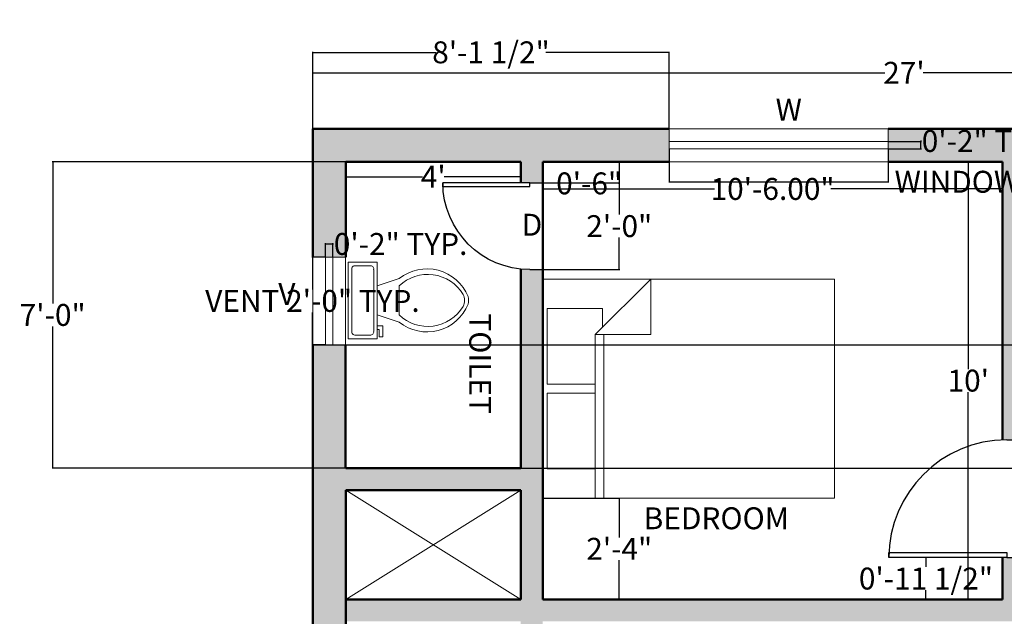
# Model space of a CAD drawing. Units: inches. Extents: x -53 to 395, y -10 to 410.
# Tile 2 of 3: x -53 to 217, y 247 to 410. Entities that reach past the tile are written whole.
import ezdxf

# ---------------------------------------------------------------- set-up
doc = ezdxf.new("R2010")
doc.units = ezdxf.units.IN
doc.header["$MEASUREMENT"] = 0
for name, color, linetype, lineweight in [('A-ANNO-DIMS', 2, 'Continuous', 18), ('A-ANNO-TEXT', 7, 'Continuous', 18), ('A-AREA-IDEN', 7, 'Continuous', 25), ('A-DOOR', 4, 'Continuous', 25), ('A-FLOR-FIXT', 9, 'Continuous', 20), ('A-FLOR-OPEN', 7, 'Continuous', 18), ('A-FURN', 8, 'Continuous', 18), ('A-GLAZ', 5, 'Continuous', 18), ('A-WALL', 7, 'Continuous', 50)]:
    doc.layers.add(name, color=color, linetype=linetype, lineweight=lineweight)
doc.layers.add('A-WALL-PATT', color=219, linetype='Continuous', lineweight=13, true_color=0x642165)
doc.styles.get("Standard").update_dxf_attribs({"font": 'arial.ttf'})
doc.dimstyles.get("Standard").update_dxf_attribs({"dimtxt": 6, "dimasz": 0.18, "dimexe": 0.18, "dimexo": 0.0625, "dimgap": 0.09, "dimtad": 0, "dimtih": 1, "dimtoh": 1, "dimzin": 0, "dimdsep": 46, "dimlunit": 3, "dimtxsty": 'Standard', "dimcen": 0.09, "dimadec": 0, "dimazin": 0, "dimtfac": 1, "dimtofl": 0, "dimtmove": 0, "dimatfit": 3, "dimfxl": 1, "dimtolj": 1, "dimtzin": 0, "dimarcsym": 0})

# ---------------------------------------------------------------- blocks, each defined once
blk = doc.blocks.new('*U2')
for p, q in [((0, 0), (0, -6)), ((40, 0), (40, -6))]:
    blk.add_line(p, q)
blk.add_lwpolyline([(0, 0), (0, 40), (1.75, 40), (1.75, 0)], close=True)
blk.add_arc((0, 0), 40, 0, 90)
blk = doc.blocks.new('Bed - Queen')
for p, q in [((0, -80.00003), (0, 0)), ((0, 0), (59.99999, 0)), ((59.99999, 0), (59.99999, -80.00003)), ((7.99999, -1.2), (28.79998, -1.2)), ((7.99999, -14.4), (7.99999, -1.2)), ((28.79998, -1.2), (28.79998, -14.4)), ((31.19999, -1.2), (51.99999, -1.2)), ((31.19999, -14.4), (31.19999, -1.2)), ((51.99999, -1.2), (51.99999, -16.4)), ((0, -14.4), (44.8, -14.4)), ((59.99999, -29.6), (44.8, -14.4)), ((44.8, -14.4), (44.8, -29.6)), ((44.8, -16.8), (0, -16.8)), ((51.99999, -16.4), (46.79936, -16.4)), ((44.8, -29.6), (59.99999, -29.6)), ((59.99999, -80.00003), (0, -80.00003))]:
    blk.add_line(p, q)
blk = doc.blocks.new('*U7')
for p, q in [((9.5, -6), (9.5, -2)), ((-8, -8.5), (-8, -8)), ((-7, -8), (-7, -9.5)), ((-4, -8), (-6, -14)), ((4, -8), (6, -14)), ((-10, -8.5), (-8, -8.5)), ((-10, -9.5), (-10, -8.5)), ((-7, -9.5), (-10, -9.5)), ((4, -14), (-4, -14))]:
    blk.add_line(p, q)
blk.add_lwpolyline([(10.5, -8), (10.5, 0), (-10.5, 0), (-10.5, -8)], close=True)
for points in [[(-9.5, -2), (-9.5, -6)], [(8.5, -1), (-8.5, -1)], [(-8.5, -7), (8.5, -7)]]:
    blk.add_lwpolyline(points)
for centre, radius, start, end in [((-8.62, -1.88), 0.884, 81.8699, 188.1301), ((8.62, -1.88), 0.884, 351.8699, 98.1301), ((-8.62, -6.12), 0.884, 171.8699, 278.1301), ((8.62, -6.12), 0.884, 261.8699, 8.1301), ((3.52, -21.58), 12.17, 141.4691, 247.9714), ((4.2, -21.82), 11.33, 136.3677, 238.9468), ((-3.52, -21.58), 12.17, 292.0284, 38.5307), ((-4.2, -21.82), 11.33, 301.053, 43.6321), ((0, -27.88), 4, 245.7318, 294.2682), ((0, -29), 4, 254.8605, 285.1395)]:
    blk.add_arc(centre, radius, start, end)
blk = doc.blocks.new('*D8')
at = {"layer": 'A-ANNO-DIMS', "color": 0, "lineweight": -2, "transparency": 16777216}
for p, q in [((27.48, 380.19), (27.48, 395.67)), ((27.66, 395.49), (184.25, 395.49)), ((351.3, 395.49), (194.72, 395.49)), ((351.48, 380.19), (351.48, 395.67))]:
    blk.add_line(p, q, dxfattribs=at)
at = {"layer": 'A-ANNO-DIMS', "color": 0, "transparency": 16777216}
for points in [[(27.66, 395.52), (27.66, 395.46), (27.48, 395.49)], [(351.3, 395.52), (351.3, 395.46), (351.48, 395.49)]]:
    blk.add_solid(points, dxfattribs=at)
at = {"layer": 'Defpoints', "color": 0, "transparency": 16777216}
for p in [(351.48, 395.49), (27.48, 380.13), (351.48, 380.13)]:
    blk.add_point(p, dxfattribs=at)
at = {"layer": 'A-ANNO-DIMS', "color": 0, "transparency": 16777216, "insert": (189.48, 395.49), "char_height": 6, "attachment_point": 5}
blk.add_mtext("\\A1;27'", dxfattribs=at)
blk = doc.blocks.new('*D17')
at = {"layer": 'A-ANNO-DIMS', "color": 0, "lineweight": -2, "transparency": 16777216}
for p, q in [((36.48, 369.82), (36.48, 366.83)), ((84.48, 369.82), (84.48, 366.83)), ((36.66, 367.01), (57.51, 367.01)), ((84.3, 367.01), (63.45, 367.01))]:
    blk.add_line(p, q, dxfattribs=at)
at = {"layer": 'A-ANNO-DIMS', "color": 0, "transparency": 16777216}
for points in [[(36.66, 367.04), (36.66, 366.98), (36.48, 367.01)], [(84.3, 367.04), (84.3, 366.98), (84.48, 367.01)]]:
    blk.add_solid(points, dxfattribs=at)
at = {"layer": 'Defpoints', "color": 0, "transparency": 16777216}
for p in [(36.48, 369.89), (84.48, 369.89), (84.48, 367.01)]:
    blk.add_point(p, dxfattribs=at)
at = {"layer": 'A-ANNO-DIMS', "color": 0, "transparency": 16777216, "insert": (60.48, 367.01), "char_height": 6, "attachment_point": 5}
blk.add_mtext("\\A1;4'", dxfattribs=at)
blk = doc.blocks.new('*D18')
at = {"layer": 'A-ANNO-DIMS', "color": 0, "lineweight": -2, "transparency": 16777216}
for p, q in [((90.48, 371.06), (90.48, 363.48)), ((216.48, 371.06), (216.48, 363.48)), ((90.66, 363.66), (137.54, 363.66)), ((216.3, 363.66), (169.42, 363.66))]:
    blk.add_line(p, q, dxfattribs=at)
at = {"layer": 'A-ANNO-DIMS', "color": 0, "transparency": 16777216}
for points in [[(90.66, 363.69), (90.66, 363.63), (90.48, 363.66)], [(216.3, 363.69), (216.3, 363.63), (216.48, 363.66)]]:
    blk.add_solid(points, dxfattribs=at)
at = {"layer": 'Defpoints', "color": 0, "transparency": 16777216}
for p in [(90.48, 371.13), (216.48, 371.13), (216.48, 363.66)]:
    blk.add_point(p, dxfattribs=at)
at = {"layer": 'A-ANNO-DIMS', "color": 0, "transparency": 16777216, "insert": (153.48, 363.66), "char_height": 6, "attachment_point": 5}
blk.add_mtext('\\A1;10\'-6.00"', dxfattribs=at)
blk = doc.blocks.new('*D19')
at = {"layer": 'A-ANNO-DIMS', "color": 0, "lineweight": -2, "transparency": 16777216}
for p, q in [((216.42, 371.13), (206.94, 371.13)), ((207.12, 370.95), (207.12, 314.28)), ((207.12, 251.31), (207.12, 307.97)), ((216.42, 251.13), (206.94, 251.13))]:
    blk.add_line(p, q, dxfattribs=at)
at = {"layer": 'A-ANNO-DIMS', "color": 0, "transparency": 16777216}
for points in [[(207.09, 370.95), (207.15, 370.95), (207.12, 371.13)], [(207.09, 251.31), (207.15, 251.31), (207.12, 251.13)]]:
    blk.add_solid(points, dxfattribs=at)
at = {"layer": 'Defpoints', "color": 0, "transparency": 16777216}
for p in [(207.12, 371.13), (216.48, 371.13), (216.48, 251.13)]:
    blk.add_point(p, dxfattribs=at)
at = {"layer": 'A-ANNO-DIMS', "color": 0, "transparency": 16777216, "insert": (207.12, 311.13), "char_height": 6, "attachment_point": 5}
blk.add_mtext("\\A1;10'", dxfattribs=at)
blk = doc.blocks.new('WIN-GLASS-60IN')
for points in [[(60, 2), (0, 2)], [(60, 0), (0, 0)]]:
    blk.add_lwpolyline(points)
blk = doc.blocks.new('VENT-GLASS-24IN')
for points in [[(0, 24), (0, 0)], [(2, 24), (2, 0)]]:
    blk.add_lwpolyline(points)
blk = doc.blocks.new('*D25')
at = {"layer": 'A-ANNO-DIMS', "color": 0, "lineweight": -2, "transparency": 16777216}
for p, q in [((125.13, 374.56), (125.13, 365.45)), ((185.13, 374.56), (185.13, 365.45)), ((125.31, 365.63), (184.95, 365.63)), ((185.13, 365.63), (185.31, 365.63))]:
    blk.add_line(p, q, dxfattribs=at)
at = {"layer": 'A-ANNO-DIMS', "color": 0, "transparency": 16777216}
for points in [[(125.31, 365.66), (125.31, 365.6), (125.13, 365.63)], [(184.95, 365.66), (184.95, 365.6), (185.13, 365.63)]]:
    blk.add_solid(points, dxfattribs=at)
at = {"layer": 'Defpoints', "color": 0, "transparency": 16777216}
for p in [(125.13, 374.63), (185.13, 374.63), (185.13, 365.63)]:
    blk.add_point(p, dxfattribs=at)
at = {"layer": 'A-ANNO-DIMS', "color": 0, "transparency": 16777216, "insert": (223.36, 365.63), "char_height": 6, "attachment_point": 5}
blk.add_mtext('\\A1;WINDOW 5\'-0" TYP.', dxfattribs=at)
blk = doc.blocks.new('*D26')
at = {"layer": 'A-ANNO-DIMS', "color": 0, "lineweight": -2, "transparency": 16777216}
for p, q in [((185.19, 376.63), (194.31, 376.63)), ((194.13, 376.63), (194.13, 376.81)), ((194.13, 376.81), (194.31, 376.81)), ((194.13, 374.81), (194.13, 376.45)), ((185.19, 374.63), (194.31, 374.63))]:
    blk.add_line(p, q, dxfattribs=at)
at = {"layer": 'A-ANNO-DIMS', "color": 0, "transparency": 16777216}
for points in [[(194.1, 376.45), (194.16, 376.45), (194.13, 376.63)], [(194.1, 374.81), (194.16, 374.81), (194.13, 374.63)]]:
    blk.add_solid(points, dxfattribs=at)
at = {"layer": 'Defpoints', "color": 0, "transparency": 16777216}
for p in [(185.13, 376.63), (194.13, 376.63), (185.13, 374.63)]:
    blk.add_point(p, dxfattribs=at)
at = {"layer": 'A-ANNO-DIMS', "color": 0, "transparency": 16777216, "insert": (212.68, 376.81), "char_height": 6, "attachment_point": 5}
blk.add_mtext('\\A1;0\'-2" TYP.', dxfattribs=at)
blk = doc.blocks.new('*D29')
at = {"layer": 'A-ANNO-DIMS', "color": 0, "lineweight": -2, "transparency": 16777216}
for p, q in [((30.92, 344.98), (27.2, 344.98)), ((27.38, 344.8), (27.38, 336.13)), ((27.38, 321.16), (27.38, 329.82)), ((30.92, 320.98), (27.2, 320.98))]:
    blk.add_line(p, q, dxfattribs=at)
at = {"layer": 'A-ANNO-DIMS', "color": 0, "transparency": 16777216}
for points in [[(27.35, 344.8), (27.41, 344.8), (27.38, 344.98)], [(27.35, 321.16), (27.41, 321.16), (27.38, 320.98)]]:
    blk.add_solid(points, dxfattribs=at)
at = {"layer": 'Defpoints', "color": 0, "transparency": 16777216}
for p in [(27.38, 344.98), (30.98, 344.98), (30.98, 320.98)]:
    blk.add_point(p, dxfattribs=at)
at = {"layer": 'A-ANNO-DIMS', "color": 0, "transparency": 16777216, "insert": (27.38, 332.98), "char_height": 6, "attachment_point": 5}
blk.add_mtext('\\A1;VENT 2\'-0" TYP.', dxfattribs=at)
blk = doc.blocks.new('*D30')
at = {"layer": 'A-ANNO-DIMS', "color": 0, "lineweight": -2, "transparency": 16777216}
for p, q in [((30.98, 345.04), (30.98, 348.76)), ((31.16, 348.58), (32.8, 348.58)), ((32.98, 345.04), (32.98, 348.76)), ((32.98, 348.58), (33.16, 348.58))]:
    blk.add_line(p, q, dxfattribs=at)
at = {"layer": 'A-ANNO-DIMS', "color": 0, "transparency": 16777216}
for points in [[(31.16, 348.61), (31.16, 348.55), (30.98, 348.58)], [(32.8, 348.61), (32.8, 348.55), (32.98, 348.58)]]:
    blk.add_solid(points, dxfattribs=at)
at = {"layer": 'Defpoints', "color": 0, "transparency": 16777216}
for p in [(32.98, 348.58), (30.98, 344.98), (32.98, 344.98)]:
    blk.add_point(p, dxfattribs=at)
at = {"layer": 'A-ANNO-DIMS', "color": 0, "transparency": 16777216, "insert": (51.54, 348.58), "char_height": 6, "attachment_point": 5}
blk.add_mtext('\\A1;0\'-2" TYP.', dxfattribs=at)
blk = doc.blocks.new('*D33')
at = {"layer": 'A-ANNO-DIMS', "color": 0, "lineweight": -2, "transparency": 16777216}
for p, q in [((36.42, 371.13), (-44, 371.13)), ((-43.82, 370.95), (-43.82, 332.28)), ((-43.82, 287.31), (-43.82, 325.97)), ((36.42, 287.13), (-44, 287.13))]:
    blk.add_line(p, q, dxfattribs=at)
at = {"layer": 'A-ANNO-DIMS', "color": 0, "transparency": 16777216}
for points in [[(-43.85, 370.95), (-43.79, 370.95), (-43.82, 371.13)], [(-43.85, 287.31), (-43.79, 287.31), (-43.82, 287.13)]]:
    blk.add_solid(points, dxfattribs=at)
at = {"layer": 'Defpoints', "color": 0, "transparency": 16777216}
for p in [(-43.82, 371.13), (36.48, 371.13), (36.48, 287.13)]:
    blk.add_point(p, dxfattribs=at)
at = {"layer": 'A-ANNO-DIMS', "color": 0, "transparency": 16777216, "insert": (-43.82, 329.13), "char_height": 6, "attachment_point": 5}
blk.add_mtext('\\A1;7\'-0"', dxfattribs=at)
blk = doc.blocks.new('*D42')
at = {"layer": 'A-ANNO-DIMS', "color": 0, "lineweight": -2, "transparency": 16777216}
for p, q in [((27.48, 380.19), (27.48, 401.28)), ((27.66, 401.1), (61.25, 401.1)), ((124.95, 401.1), (91.36, 401.1)), ((125.13, 380.19), (125.13, 401.28))]:
    blk.add_line(p, q, dxfattribs=at)
at = {"layer": 'A-ANNO-DIMS', "color": 0, "transparency": 16777216}
for points in [[(27.66, 401.13), (27.66, 401.07), (27.48, 401.1)], [(124.95, 401.13), (124.95, 401.07), (125.13, 401.1)]]:
    blk.add_solid(points, dxfattribs=at)
at = {"layer": 'Defpoints', "color": 0, "transparency": 16777216}
for p in [(125.13, 401.1), (27.48, 380.13), (125.13, 380.13)]:
    blk.add_point(p, dxfattribs=at)
at = {"layer": 'A-ANNO-DIMS', "color": 0, "transparency": 16777216, "insert": (76.31, 401.1), "char_height": 6, "attachment_point": 5}
blk.add_mtext('\\A1;8\'-1 1/2"', dxfattribs=at)
blk = doc.blocks.new('*D46')
at = {"layer": 'A-ANNO-DIMS', "color": 0, "lineweight": -2, "transparency": 16777216}
for p, q in [((27.55, 320.98), (372.64, 320.98)), ((372.46, 320.8), (372.46, 307.21)), ((372.46, 287.31), (372.46, 300.9)), ((36.55, 287.13), (372.64, 287.13))]:
    blk.add_line(p, q, dxfattribs=at)
at = {"layer": 'A-ANNO-DIMS', "color": 0, "transparency": 16777216}
for points in [[(372.43, 320.8), (372.49, 320.8), (372.46, 320.98)], [(372.43, 287.31), (372.49, 287.31), (372.46, 287.13)]]:
    blk.add_solid(points, dxfattribs=at)
at = {"layer": 'Defpoints', "color": 0, "transparency": 16777216}
for p in [(27.48, 320.98), (372.46, 320.98), (36.48, 287.13)]:
    blk.add_point(p, dxfattribs=at)
at = {"layer": 'A-ANNO-DIMS', "color": 0, "transparency": 16777216, "insert": (372.46, 304.05), "char_height": 6, "attachment_point": 5}
blk.add_mtext('\\A1;2\'-10"', dxfattribs=at)
blk = doc.blocks.new('*D48')
at = {"layer": 'A-ANNO-DIMS', "color": 0, "lineweight": -2, "transparency": 16777216}
for p, q in [((90.55, 365.37), (111.64, 365.37)), ((111.46, 365.19), (111.46, 356.63)), ((111.46, 341.76), (111.46, 350.32)), ((90.55, 341.58), (111.64, 341.58))]:
    blk.add_line(p, q, dxfattribs=at)
at = {"layer": 'A-ANNO-DIMS', "color": 0, "transparency": 16777216}
for points in [[(111.43, 365.19), (111.49, 365.19), (111.46, 365.37)], [(111.43, 341.76), (111.49, 341.76), (111.46, 341.58)]]:
    blk.add_solid(points, dxfattribs=at)
at = {"layer": 'Defpoints', "color": 0, "transparency": 16777216}
for p in [(90.48, 365.37), (90.48, 341.58), (111.46, 341.58)]:
    blk.add_point(p, dxfattribs=at)
at = {"layer": 'A-ANNO-DIMS', "color": 0, "transparency": 16777216, "insert": (111.46, 353.47), "char_height": 6, "attachment_point": 5}
blk.add_mtext('\\A1;2\'-0"', dxfattribs=at)
blk = doc.blocks.new('*D49')
at = {"layer": 'A-ANNO-DIMS', "color": 0, "lineweight": -2, "transparency": 16777216}
for p, q in [((90.55, 371.13), (111.64, 371.13)), ((111.46, 370.95), (111.46, 365.55)), ((90.55, 365.37), (111.64, 365.37)), ((111.46, 365.19), (111.28, 365.19)), ((111.46, 365.37), (111.46, 365.19))]:
    blk.add_line(p, q, dxfattribs=at)
at = {"layer": 'A-ANNO-DIMS', "color": 0, "transparency": 16777216}
for points in [[(111.43, 370.95), (111.49, 370.95), (111.46, 371.13)], [(111.43, 365.55), (111.49, 365.55), (111.46, 365.37)]]:
    blk.add_solid(points, dxfattribs=at)
at = {"layer": 'Defpoints', "color": 0, "transparency": 16777216}
for p in [(90.48, 371.13), (90.48, 365.37), (111.46, 365.37)]:
    blk.add_point(p, dxfattribs=at)
at = {"layer": 'A-ANNO-DIMS', "color": 0, "transparency": 16777216, "insert": (103.21, 365.19), "char_height": 6, "attachment_point": 5}
blk.add_mtext('\\A1;0\'-6"', dxfattribs=at)
blk = doc.blocks.new('*D51')
at = {"layer": 'A-ANNO-DIMS', "color": 0, "lineweight": -2, "transparency": 16777216}
for p, q in [((216.42, 262.63), (195.33, 262.63)), ((195.51, 262.45), (195.51, 260.07)), ((195.51, 251.31), (195.51, 253.69)), ((216.42, 251.13), (195.33, 251.13))]:
    blk.add_line(p, q, dxfattribs=at)
at = {"layer": 'A-ANNO-DIMS', "color": 0, "transparency": 16777216}
for points in [[(195.48, 262.45), (195.54, 262.45), (195.51, 262.63)], [(195.48, 251.31), (195.54, 251.31), (195.51, 251.13)]]:
    blk.add_solid(points, dxfattribs=at)
at = {"layer": 'Defpoints', "color": 0, "transparency": 16777216}
for p in [(195.51, 262.63), (216.48, 262.63), (216.48, 251.13)]:
    blk.add_point(p, dxfattribs=at)
at = {"layer": 'A-ANNO-DIMS', "color": 0, "transparency": 16777216, "insert": (195.51, 256.88), "char_height": 6, "attachment_point": 5}
blk.add_mtext('\\A1;0\'-11 1/2"', dxfattribs=at)
blk = doc.blocks.new('*D61')
at = {"layer": 'A-ANNO-DIMS', "color": 0, "lineweight": -2, "transparency": 16777216}
for p, q in [((90.54, 278.92), (111.64, 278.92)), ((111.46, 278.74), (111.46, 268.13)), ((111.46, 251.31), (111.46, 261.92)), ((90.55, 251.13), (111.64, 251.13))]:
    blk.add_line(p, q, dxfattribs=at)
at = {"layer": 'A-ANNO-DIMS', "color": 0, "transparency": 16777216}
for points in [[(111.49, 278.74), (111.43, 278.74), (111.46, 278.92)], [(111.49, 251.31), (111.43, 251.31), (111.46, 251.13)]]:
    blk.add_solid(points, dxfattribs=at)
at = {"layer": 'Defpoints', "color": 0, "transparency": 16777216}
for p in [(90.48, 278.92), (90.48, 251.13), (111.46, 251.13)]:
    blk.add_point(p, dxfattribs=at)
at = {"layer": 'A-ANNO-DIMS', "color": 0, "transparency": 16777216, "insert": (111.46, 265.03), "char_height": 6, "attachment_point": 5}
blk.add_mtext('\\A1;2\'-4"', dxfattribs=at)

msp = doc.modelspace()

# ---------------------------------------------------------------- hatches: boundary and pattern name
at = {"layer": 'A-WALL-PATT'}
h = msp.add_hatch(color=256, dxfattribs=at)
h.dxf.hatch_style = 1
h.paths.add_polyline_path([(36.483, 371.127), (84.483, 371.127), (84.483, 365.369), (86.914, 365.369), (90.483, 365.369), (90.483, 371.127), (125.127, 371.127), (125.127, 380.127), (27.483, 380.127), (27.483, 344.976), (36.483, 344.976)])
h.paths.add_polyline_path([(256.886, 380.127), (185.127, 380.127), (185.127, 371.127), (216.483, 371.127), (216.483, 294.874, -0.0089901), (217.643, 294.895), (222.483, 294.895), (222.483, 371.127), (256.886, 371.127)])
h.paths.add_polyline_path([(351.483, 380.127), (316.886, 380.127), (316.886, 371.127), (342.483, 371.127), (342.483, 370.595), (342.483, 357.645), (351.483, 357.645)])
h.paths.add_polyline_path([(351.483, 297.645), (342.483, 297.645), (342.483, 246.678), (351.483, 246.678)])
h.paths.add_polyline_path([(351.483, 186.678), (342.483, 186.678), (342.483, 174.127), (263.983, 174.127), (263.983, 158.936), (268.991, 158.936), (269.483, 158.936), (269.483, 163.127), (351.483, 163.127)])
h.paths.add_polyline_path([(90.483, 245.127), (84.483, 245.127), (84.483, 173.127), (90.483, 173.127)])
h = msp.add_hatch(color=256, dxfattribs=at)
h.dxf.hatch_style = 1
h.paths.add_polyline_path([(90.483, 278.924), (90.482, 278.924), (90.482, 338.924), (90.482, 341.579), (86.914, 341.579, -0.0256023), (84.483, 341.703), (84.483, 287.127), (36.467, 287.127), (36.467, 320.976), (27.483, 320.976), (27.483, 224.19), (36.483, 224.19), (36.483, 281.127), (84.483, 281.127), (84.483, 251.127), (36.483, 251.127), (36.483, 245.127), (222.483, 245.127), (222.483, 262.629), (217.643, 262.629), (216.483, 262.629), (216.483, 251.127), (90.483, 251.127)])

# ---------------------------------------------------------------- linework, layer by layer
at = {"layer": 'A-FLOR-OPEN'}
for p, q in [((36.483, 281.127), (84.483, 251.127)), ((36.483, 251.127), (84.483, 281.127))]:
    msp.add_line(p, q, dxfattribs=at)
at = {"layer": 'A-GLAZ'}
for points in [[(125.127, 380.127), (185.127, 380.127), (185.127, 371.127), (125.127, 371.127)], [(27.467, 344.976), (36.467, 344.976), (36.467, 320.976), (27.467, 320.976)]]:
    msp.add_lwpolyline(points, close=True, dxfattribs=at)
at = {"layer": 'A-WALL'}
for p, q in [((27.467, 344.976), (27.483, 344.976)), ((36.467, 320.976), (36.483, 320.976))]:
    msp.add_line(p, q, dxfattribs=at)
for points in [[(125.127, 380.127), (27.483, 380.127), (27.483, 344.976)], [(256.886, 380.127), (185.127, 380.127)], [(36.483, 371.127), (36.483, 344.976)], [(84.483, 371.127), (36.483, 371.127)], [(84.483, 371.127), (84.483, 365.369)], [(84.483, 371.127), (84.483, 365.369)], [(90.483, 371.127), (90.483, 251.127)], [(125.127, 371.127), (90.483, 371.127)], [(216.483, 371.127), (185.127, 371.127)], [(216.483, 294.874), (216.483, 371.127)], [(84.483, 341.703), (84.483, 287.127)], [(84.483, 341.703), (84.483, 287.127)], [(27.483, 320.976), (27.483, 224.19)], [(36.467, 320.976), (36.467, 287.127)], [(84.483, 287.127), (36.483, 287.127)], [(84.483, 281.127), (36.483, 281.127)], [(36.483, 281.127), (36.483, 224.19)], [(84.483, 281.127), (84.483, 251.127)], [(84.483, 281.127), (84.483, 251.127)], [(216.483, 251.127), (216.483, 262.629)], [(84.483, 251.127), (36.483, 251.127)], [(216.483, 251.127), (90.483, 251.127)]]:
    msp.add_lwpolyline(points, dxfattribs=at)

# ---------------------------------------------------------------- block references
at = {"layer": 'A-DOOR', "rotation": 90}
for p, xscale, yscale, zscale in [((86.914, 365.369), -0.5947469315104942, 0.5947469315104942, 0.5947469315104942), ((217.643, 262.629), 0.8066612292799318, 0.8066612292799318, 0.8066612292799318)]:
    msp.add_blockref('*U2', p, dxfattribs=dict(at, xscale=xscale, yscale=yscale, zscale=zscale))
at = {"layer": 'A-FLOR-FIXT', "rotation": 90.00000000000003}
msp.add_blockref('*U7', (37.158, 333.12), dxfattribs=at)
at = {"layer": 'A-FURN', "rotation": 90}
msp.add_blockref('Bed - Queen', (90.482, 278.924), dxfattribs=at)
at = {"layer": 'A-GLAZ'}
for name, p in [('WIN-GLASS-60IN', (125.127, 374.627)), ('VENT-GLASS-24IN', (30.983, 320.976))]:
    msp.add_blockref(name, p, dxfattribs=at)

# ---------------------------------------------------------------- texts
at = {"layer": 'A-ANNO-TEXT', "char_height": 6, "attachment_point": 1}
for s, insert in [('W', (154.323, 388.399)), ('D', (84.736, 356.851)), ('V', (18.005, 337.875))]:
    msp.add_mtext_dynamic_manual_height_columns(s, width=74.47502, gutter_width=1, heights=[0], dxfattribs=dict(at, insert=insert))
at = {"layer": 'A-AREA-IDEN', "insert": (76.353, 329.559), "char_height": 6, "attachment_point": 1, "rotation": 270}
msp.add_mtext_dynamic_manual_height_columns('TOILET', width=74.47502, gutter_width=1, heights=[0], dxfattribs=at)
at = {"layer": 'A-AREA-IDEN', "insert": (118.162, 276.397), "char_height": 6, "attachment_point": 1}
msp.add_mtext_dynamic_manual_height_columns('BEDROOM', width=74.47502, gutter_width=1, heights=[0], dxfattribs=at)

# ---------------------------------------------------------------- dimensions: what is measured, and where the dimension line sits
at = {"layer": 'A-ANNO-DIMS'}
for base, p1, p2, override, picture, middle in [((125.127, 401.102), (27.483, 380.127), (125.127, 380.127), {"dimdec": 1, "dimlfac": 1, "dimrnd": 0, "dimzin": 1, "dimdsep": 46, "dimlunit": 4, "dimfrac": 2}, '*D42', (76.305, 401.102)), ((351.483, 395.485), (27.483, 380.127), (351.483, 380.127), {"dimclrd": 0, "dimclre": 0, "dimclrt": 0}, '*D8', (189.483, 395.485)), ((84.483, 367.006), (36.483, 369.885), (84.483, 369.885), {"dimclrd": 0, "dimclre": 0, "dimclrt": 0}, '*D17', (60.483, 367.006)), ((216.483, 363.659), (90.483, 371.127), (216.483, 371.127), {"dimclrd": 0, "dimclre": 0, "dimclrt": 0}, '*D18', (153.483, 363.659))]:
    dim = msp.add_linear_dim(base=base, p1=p1, p2=p2, dimstyle='Standard', override=override, dxfattribs=at)
    dim.commit()
    dim.dimension.update_dxf_attribs({"geometry": picture, "text_midpoint": middle})
for base, p1, p2, text, picture, middle in [((194.127, 376.627), (185.127, 374.627), (185.127, 376.627), '<> TYP.', '*D26', (212.684, 376.807)), ((27.383, 344.976), (30.983, 320.976), (30.983, 344.976), 'VENT <> TYP.', '*D29', (27.383, 332.976))]:
    dim = msp.add_linear_dim(base=base, p1=p1, p2=p2, angle=90, text=text, dimstyle='Standard', override={"dimdec": 1, "dimlfac": 1, "dimrnd": 0, "dimzin": 1, "dimdsep": 46, "dimlunit": 4, "dimfrac": 2}, dxfattribs=at)
    dim.commit()
    dim.dimension.update_dxf_attribs({"geometry": picture, "text_midpoint": middle})
for base, p1, p2, text, picture, middle in [((185.127, 365.627), (125.127, 374.627), (185.127, 374.627), 'WINDOW <> TYP.', '*D25', (223.36, 365.627)), ((32.983, 348.576), (30.983, 344.976), (32.983, 344.976), '<> TYP.', '*D30', (51.539, 348.576))]:
    dim = msp.add_linear_dim(base=base, p1=p1, p2=p2, text=text, dimstyle='Standard', override={"dimdec": 1, "dimlfac": 1, "dimrnd": 0, "dimzin": 1, "dimdsep": 46, "dimlunit": 4, "dimfrac": 2}, dxfattribs=at)
    dim.commit()
    dim.dimension.update_dxf_attribs({"geometry": picture, "text_midpoint": middle})
for base, p1, p2, angle, override, picture, middle in [((-43.817, 371.127), (36.483, 287.127), (36.483, 371.127), 90, {"dimdec": 1, "dimlfac": 1, "dimrnd": 0, "dimzin": 1, "dimdsep": 46, "dimlunit": 4, "dimfrac": 2}, '*D33', (-43.817, 329.127)), ((111.458, 365.369), (90.483, 371.127), (90.483, 365.369), 270, {"dimdec": 1, "dimlfac": 1, "dimrnd": 0, "dimzin": 1, "dimdsep": 46, "dimlunit": 4, "dimfrac": 2}, '*D49', (103.213, 365.189)), ((207.116, 371.127), (216.483, 251.127), (216.483, 371.127), 90, {"dimclrd": 0, "dimclre": 0, "dimclrt": 0}, '*D19', (207.116, 311.127)), ((111.458, 341.579), (90.483, 365.369), (90.483, 341.579), 270, {"dimdec": 1, "dimlfac": 1, "dimrnd": 0, "dimzin": 1, "dimdsep": 46, "dimlunit": 4, "dimfrac": 2}, '*D48', (111.458, 353.474)), ((372.458, 320.976), (36.483, 287.127), (27.483, 320.976), 90, {"dimdec": 1, "dimlfac": 1, "dimrnd": 0, "dimzin": 1, "dimdsep": 46, "dimlunit": 4, "dimfrac": 2}, '*D46', (372.458, 304.052)), ((111.458, 251.128), (90.482, 278.924), (90.483, 251.127), 270.00125, {"dimdec": 1, "dimlfac": 1, "dimrnd": 0, "dimzin": 1, "dimdsep": 46, "dimlunit": 4, "dimfrac": 2}, '*D61', (111.457, 265.026)), ((195.508, 262.629), (216.483, 251.127), (216.483, 262.629), 90, {"dimdec": 1, "dimlfac": 1, "dimrnd": 0, "dimzin": 1, "dimdsep": 46, "dimlunit": 4, "dimfrac": 2}, '*D51', (195.508, 256.878))]:
    dim = msp.add_linear_dim(base=base, p1=p1, p2=p2, angle=angle, dimstyle='Standard', override=override, dxfattribs=at)
    dim.commit()
    dim.dimension.update_dxf_attribs({"geometry": picture, "text_midpoint": middle})

doc.saveas('drawing.dxf')
